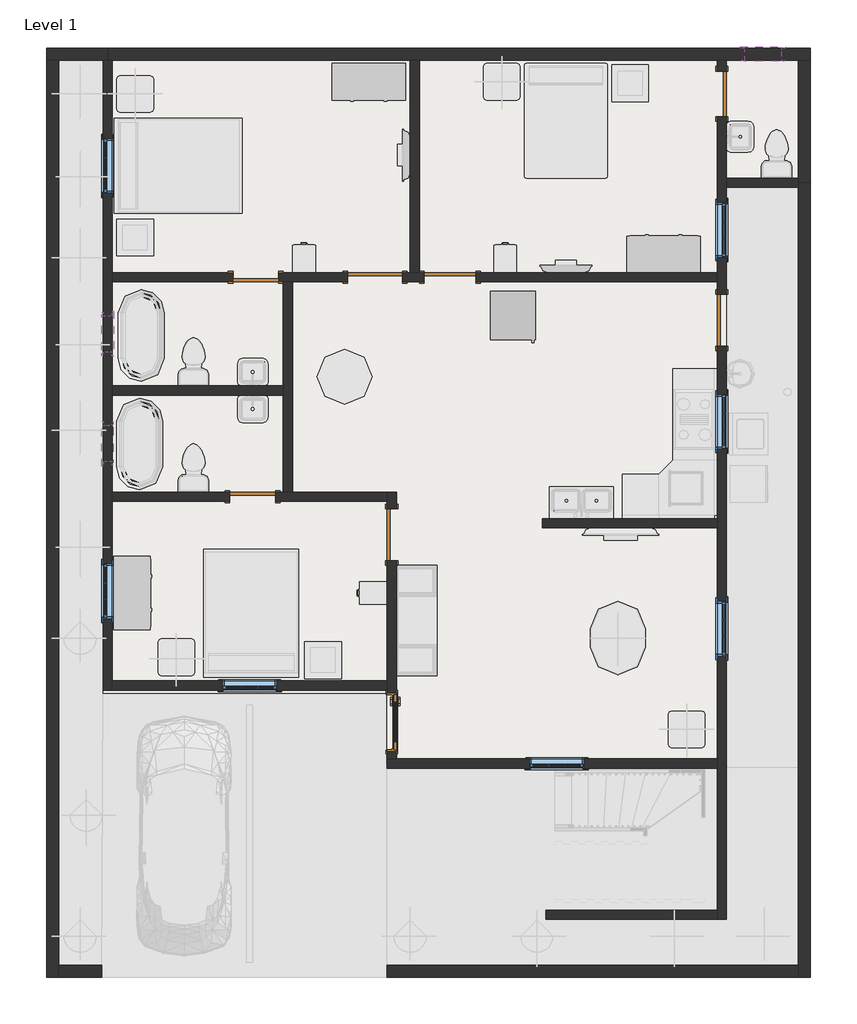
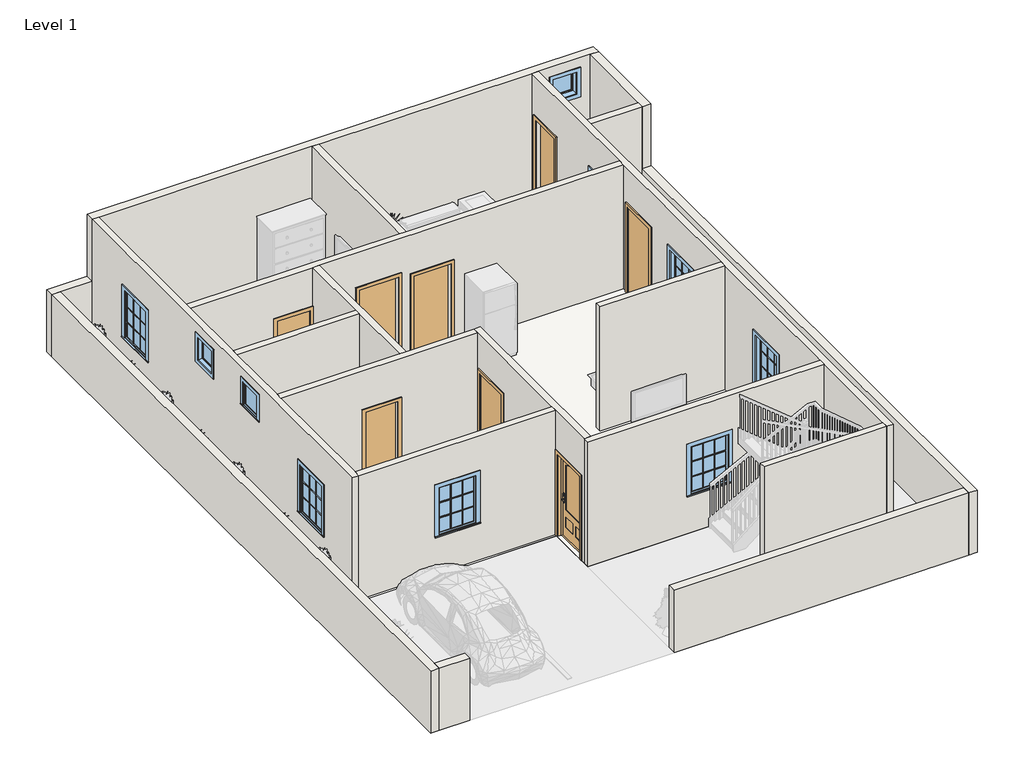
# One storey, part 1 of 3: 20 walls, 10 windows, 8 doors, 1 slab.
"""IFC4 building model written with IfcOpenShell, lengths in millimetres."""

from ifc_helpers import new_model, si_unit, frame, origin, origin_with_axes, place, context, project, spatial, polyline, outline, extrude, faceted_brep, transform, mapped, element, save
from components import door_5d363d20, door_255cab33, door_059fdd7e, door_706f0888, door_b6e9fca3, door_16372e1c, window_5c190c7e, window_e41d21a6, window_3d781103

model = new_model("IFC4")

# Units and contexts
model_context = context("Model", 3, world=origin())
ifc_project = project(units=[si_unit("LENGTHUNIT", "METRE", prefix="MILLI")], contexts=[model_context])

# Site, building, storey
site = spatial("IfcSite", under=ifc_project)
building = spatial("IfcBuilding", under=site)
storey = spatial("IfcBuildingStorey", under=building, Name="Level 1", Elevation=0.0)

# Doors
placement = place(None, origin())
door_shape = door_5d363d20(model_context)
element("IfcDoor", 1, ObjectType="36\" x 80\"", at=placement, inside=storey, context=model_context, shape_type="MappedRepresentation", body=[
    mapped(door_shape, transform((-6677.6504019, 2135.1007235, 0.0), x_axis=(0.0, 1.0, 0.0), y_axis=(-1.0, 0.0, 0.0), z_axis=(0.0, 0.0, 1.0))),
])
door_2_shape = door_255cab33(model_context)
element("IfcDoor", 2, ObjectType="Single-Flush : 30\" x 80\"", at=placement, inside=storey, context=model_context, shape_type="MappedRepresentation", body=[
    mapped(door_2_shape, transform((-8941.4254019, 9526.5007235, 0.0), x_axis=(1.0, 0.0, 0.0), y_axis=(0.0, 1.0, 0.0), z_axis=(0.0, 0.0, 1.0))),
])
element("IfcDoor", 3, ObjectType="Single-Flush : 30\" x 80\"", at=placement, inside=storey, context=model_context, shape_type="MappedRepresentation", body=[
    mapped(door_2_shape, transform((-1194.4254019, 12574.5007235, 0.0), x_axis=(0.0, 1.0, 0.0), y_axis=(-1.0, 0.0, 0.0), z_axis=(0.0, 0.0, 1.0))),
])
door_3_shape = door_059fdd7e(model_context)
element("IfcDoor", 4, ObjectType="Single-Flush : 30\" x 80\"", at=placement, inside=storey, context=model_context, shape_type="MappedRepresentation", body=[
    mapped(door_3_shape, transform((-8992.2254019, 5882.5032847, 0.0), x_axis=(1.0, 0.0, 0.0), y_axis=(0.0, 1.0, 0.0), z_axis=(0.0, 0.0, 1.0))),
])
door_4_shape = door_706f0888(model_context)
element("IfcDoor", 5, ObjectType="Single-Flush : 34\" x 80\"", at=placement, inside=storey, context=model_context, shape_type="MappedRepresentation", body=[
    mapped(door_4_shape, transform((-5715.6254019, 9526.5007235, 0.0), x_axis=(-1.0, 0.0, 0.0), y_axis=(0.0, -1.0, 0.0), z_axis=(0.0, 0.0, 1.0))),
])
door_5_shape = door_b6e9fca3(model_context)
element("IfcDoor", 6, ObjectType="Single-Flush : 34\" x 84\"", at=placement, inside=storey, context=model_context, shape_type="MappedRepresentation", body=[
    mapped(door_5_shape, transform((-6680.8254019, 5247.5032847, 0.0), x_axis=(0.0, 1.0, 0.0), y_axis=(-1.0, 0.0, 0.0), z_axis=(0.0, 0.0, 1.0))),
])
element("IfcDoor", 7, ObjectType="Single-Flush : 34\" x 84\"", at=placement, inside=storey, context=model_context, shape_type="MappedRepresentation", body=[
    mapped(door_5_shape, transform((-1194.4254019, 8815.3007235, 0.0), x_axis=(0.0, 1.0, 0.0), y_axis=(-1.0, 0.0, 0.0), z_axis=(0.0, 0.0, 1.0))),
])
door_6_shape = door_16372e1c(model_context)
element("IfcDoor", 8, ObjectType="Single-Flush : 36\" x 84\"", at=placement, inside=storey, context=model_context, shape_type="MappedRepresentation", body=[
    mapped(door_6_shape, transform((-6960.2254019, 9526.5007235, 0.0), x_axis=(1.0, 0.0, 0.0), y_axis=(0.0, 1.0, 0.0), z_axis=(0.0, 0.0, 1.0))),
])

# Slab
element("IfcSlab", 9, ObjectType="Generic - 12\"", at=placement, inside=storey, context=model_context, shape_type="SweptSolid", body=[
    extrude(outline(polyline([(278.7745981, 13336.5007235), (278.7745981, 11025.1007235), (-1118.2254019, 11025.1007235), (-1118.2254019, 1373.1007235), (-6757.0254019, 1373.1007235), (-6757.0254019, 2617.7007235), (-11481.4254019, 2617.7007235), (-11481.4254019, 13336.5007235), (278.7745981, 13336.5007235)])), frame((0.0, 0.0, -304.8), z_axis=(0.0, 0.0, 1.0), x_axis=(1.0, 0.0, 0.0)), (0.0, 0.0, 1.0), 304.8),
])

# Walls
element("IfcWall", 10, ObjectType="Generic - 8\"", at=placement, inside=storey, context=model_context, shape_type="Brep", body=[
    faceted_brep([(75.5745981, 13133.3007235, 0.0), (75.5745981, 11177.5007235, 0.0), (75.5745981, 11101.3007235, 0.0), (75.5745981, 11101.3007235, 1524.0), (75.5745981, 11025.1007235, 1524.0), (75.5745981, 11025.1007235, 3048.0), (75.5745981, 11177.5007235, 3048.0), (75.5745981, 13133.3007235, 3048.0), (278.7745981, 13133.3007235, 0.0), (278.7745981, 13133.3007235, 3048.0), (278.7745981, 11025.1007235, 3048.0), (278.7745981, 11025.1007235, 1524.0), (278.7745981, 11101.3007235, 1524.0), (278.7745981, 11101.3007235, 0.0)], [[[0, 1, 2, 3, 4, 5, 6, 7]], [[8, 9, 10, 11, 12, 13]], [[2, 1, 0, 8, 13]], [[0, 7, 9, 8]], [[3, 2, 13, 12]], [[11, 4, 3, 12]], [[5, 4, 11, 10]], [[7, 6, 5, 10, 9]]]),
])
element("IfcWall", 11, ObjectType="Generic - 8\"", at=placement, inside=storey, context=model_context, shape_type="Brep", body=[
    faceted_brep([(-11405.2254019, 13133.3007235, 0.0), (-11329.0254019, 13133.3007235, 0.0), (-6376.0254019, 13133.3007235, 0.0), (-6223.6254019, 13133.3007235, 0.0), (-1270.6254019, 13133.3007235, 0.0), (-1118.2254019, 13133.3007235, 0.0), (75.5745981, 13133.3007235, 0.0), (278.7745981, 13133.3007235, 0.0), (278.7745981, 13133.3007235, 3048.0), (75.5745981, 13133.3007235, 3048.0), (-1118.2254019, 13133.3007235, 3048.0), (-1270.6254019, 13133.3007235, 3048.0), (-6223.6254019, 13133.3007235, 3048.0), (-6376.0254019, 13133.3007235, 3048.0), (-11329.0254019, 13133.3007235, 3048.0), (-11481.4254019, 13133.3007235, 3048.0), (-11481.4254019, 13133.3007235, 1524.0), (-11405.2254019, 13133.3007235, 1524.0), (-203.8254019, 13133.3007235, 2768.6), (-203.8254019, 13133.3007235, 2159.0), (-813.4254019, 13133.3007235, 2159.0), (-813.4254019, 13133.3007235, 2768.6), (-11405.2254019, 13336.5007235, 0.0), (-11405.2254019, 13336.5007235, 1524.0), (-11481.4254019, 13336.5007235, 1524.0), (-11481.4254019, 13336.5007235, 3048.0), (278.7745981, 13336.5007235, 3048.0), (278.7745981, 13336.5007235, 0.0), (-203.8254019, 13336.5007235, 2768.6), (-813.4254019, 13336.5007235, 2768.6), (-813.4254019, 13336.5007235, 2159.0), (-203.8254019, 13336.5007235, 2159.0)], [[[0, 1, 2, 3, 4, 5, 6, 7, 8, 9, 10, 11, 12, 13, 14, 15, 16, 17], [18, 19, 20, 21]], [[22, 23, 24, 25, 26, 27], [28, 29, 30, 31]], [[7, 6, 5, 4, 3, 2, 1, 0, 22, 27]], [[8, 7, 27, 26]], [[19, 18, 28, 31]], [[20, 19, 31, 30]], [[21, 20, 30, 29]], [[18, 21, 29, 28]], [[0, 17, 23, 22]], [[16, 24, 23, 17]], [[16, 15, 25, 24]], [[15, 14, 13, 12, 11, 10, 9, 8, 26, 25]]]),
])
element("IfcWall", 12, ObjectType="INNER 6\"", at=placement, inside=storey, context=model_context, shape_type="Brep", body=[
    faceted_brep([(-6503.0254019, 9450.3007235, 0.0), (-6147.4254019, 9450.3007235, 0.0), (-6147.4254019, 9450.3007235, 2032.0), (-5283.8254019, 9450.3007235, 2032.0), (-5283.8254019, 9450.3007235, 0.0), (-1270.6254019, 9450.3007235, 0.0), (-1270.6254019, 9450.3007235, 3048.0), (-8331.8254019, 9450.3007235, 3048.0), (-8484.2254019, 9450.3007235, 3048.0), (-11329.0254019, 9450.3007235, 3048.0), (-11329.0254019, 9450.3007235, 0.0), (-9322.4254019, 9450.3007235, 0.0), (-9322.4254019, 9450.3007235, 2032.0), (-8560.4254019, 9450.3007235, 2032.0), (-8560.4254019, 9450.3007235, 0.0), (-8484.2254019, 9450.3007235, 0.0), (-8331.8254019, 9450.3007235, 0.0), (-7417.4254019, 9450.3007235, 0.0), (-7417.4254019, 9450.3007235, 2133.6), (-6503.0254019, 9450.3007235, 2133.6), (-6147.4254019, 9602.7007235, 2032.0), (-6147.4254019, 9602.7007235, 0.0), (-6223.6254019, 9602.7007235, 0.0), (-6376.0254019, 9602.7007235, 0.0), (-6503.0254019, 9602.7007235, 0.0), (-6503.0254019, 9602.7007235, 2133.6), (-7417.4254019, 9602.7007235, 2133.6), (-7417.4254019, 9602.7007235, 0.0), (-8560.4254019, 9602.7007235, 0.0), (-8560.4254019, 9602.7007235, 2032.0), (-9322.4254019, 9602.7007235, 2032.0), (-9322.4254019, 9602.7007235, 0.0), (-11329.0254019, 9602.7007235, 0.0), (-11329.0254019, 9602.7007235, 3048.0), (-6376.0254019, 9602.7007235, 3048.0), (-6223.6254019, 9602.7007235, 3048.0), (-1270.6254019, 9602.7007235, 3048.0), (-1270.6254019, 9602.7007235, 0.0), (-5283.8254019, 9602.7007235, 0.0), (-5283.8254019, 9602.7007235, 2032.0)], [[[0, 1, 2, 3, 4, 5, 6, 7, 8, 9, 10, 11, 12, 13, 14, 15, 16, 17, 18, 19]], [[20, 21, 22, 23, 24, 25, 26, 27, 28, 29, 30, 31, 32, 33, 34, 35, 36, 37, 38, 39]], [[11, 10, 32, 31]], [[17, 16, 15, 14, 28, 27]], [[38, 37, 5, 4]], [[24, 23, 22, 21, 1, 0]], [[10, 9, 33, 32]], [[6, 5, 37, 36]], [[25, 24, 0, 19]], [[26, 25, 19, 18]], [[27, 26, 18, 17]], [[29, 28, 14, 13]], [[30, 29, 13, 12]], [[31, 30, 12, 11]], [[2, 1, 21, 20]], [[3, 2, 20, 39]], [[4, 3, 39, 38]], [[9, 8, 7, 6, 36, 35, 34, 33]]]),
])
element("IfcWall", 13, ObjectType="INNER 6\"", at=placement, inside=storey, context=model_context, shape_type="SweptSolid", body=[
    extrude(outline(polyline([(-6223.6254019, 13133.3007235), (-6223.6254019, 9602.7007235), (-6376.0254019, 9602.7007235), (-6376.0254019, 13133.3007235), (-6223.6254019, 13133.3007235)])), origin_with_axes(), (0.0, 0.0, 1.0), 3048.0),
])
element("IfcWall", 14, ObjectType="INNER 6\"", at=placement, inside=storey, context=model_context, shape_type="Brep", body=[
    faceted_brep([(-1118.2254019, 12955.5007235, 2032.0), (-1118.2254019, 12955.5007235, 0.0), (-1118.2254019, 13133.3007235, 0.0), (-1118.2254019, 13133.3007235, 3048.0), (-1118.2254019, 11177.5007235, 3048.0), (-1118.2254019, 11025.1007235, 3048.0), (-1118.2254019, -1141.4992765, 3048.0), (-1118.2254019, -1141.4992765, 0.0), (-1118.2254019, 8383.5007235, 0.0), (-1118.2254019, 8383.5007235, 2133.6), (-1118.2254019, 9247.1007235, 2133.6), (-1118.2254019, 9247.1007235, 0.0), (-1118.2254019, 11025.1007235, 0.0), (-1118.2254019, 11177.5007235, 0.0), (-1118.2254019, 12193.5007235, 0.0), (-1118.2254019, 12193.5007235, 2032.0), (-1118.2254019, 3232.7671827, 2133.6), (-1118.2254019, 4147.1671827, 2133.6), (-1118.2254019, 4147.1671827, 914.4), (-1118.2254019, 3232.7671827, 914.4), (-1118.2254019, 6671.7339531, 2133.6), (-1118.2254019, 7586.1339531, 2133.6), (-1118.2254019, 7586.1339531, 914.4), (-1118.2254019, 6671.7339531, 914.4), (-1118.2254019, 9856.7007235, 2133.6), (-1118.2254019, 10771.1007235, 2133.6), (-1118.2254019, 10771.1007235, 914.4), (-1118.2254019, 9856.7007235, 914.4), (-1270.6254019, 13133.3007235, 0.0), (-1270.6254019, 12955.5007235, 0.0), (-1270.6254019, 12955.5007235, 2032.0), (-1270.6254019, 12193.5007235, 2032.0), (-1270.6254019, 12193.5007235, 0.0), (-1270.6254019, 9602.7007235, 0.0), (-1270.6254019, 9450.3007235, 0.0), (-1270.6254019, 9247.1007235, 0.0), (-1270.6254019, 9247.1007235, 2133.6), (-1270.6254019, 8383.5007235, 2133.6), (-1270.6254019, 8383.5007235, 0.0), (-1270.6254019, 5518.7671827, 0.0), (-1270.6254019, 5366.3671827, 0.0), (-1270.6254019, 1525.5007235, 0.0), (-1270.6254019, 1373.1007235, 0.0), (-1270.6254019, -989.0992765, 0.0), (-1270.6254019, -1141.4992765, 0.0), (-1270.6254019, -1141.4992765, 3048.0), (-1270.6254019, -989.0992765, 3048.0), (-1270.6254019, 1373.1007235, 3048.0), (-1270.6254019, 1525.5007235, 3048.0), (-1270.6254019, 5366.3671827, 3048.0), (-1270.6254019, 5518.7671827, 3048.0), (-1270.6254019, 9450.3007235, 3048.0), (-1270.6254019, 9602.7007235, 3048.0), (-1270.6254019, 13133.3007235, 3048.0), (-1270.6254019, 3232.7671827, 2133.6), (-1270.6254019, 3232.7671827, 914.4), (-1270.6254019, 4147.1671827, 914.4), (-1270.6254019, 4147.1671827, 2133.6), (-1270.6254019, 6671.7339531, 2133.6), (-1270.6254019, 6671.7339531, 914.4), (-1270.6254019, 7586.1339531, 914.4), (-1270.6254019, 7586.1339531, 2133.6), (-1270.6254019, 9856.7007235, 2133.6), (-1270.6254019, 9856.7007235, 914.4), (-1270.6254019, 10771.1007235, 914.4), (-1270.6254019, 10771.1007235, 2133.6)], [[[0, 1, 2, 3, 4, 5, 6, 7, 8, 9, 10, 11, 12, 13, 14, 15], [16, 17, 18, 19], [20, 21, 22, 23], [24, 25, 26, 27]], [[28, 29, 30, 31, 32, 33, 34, 35, 36, 37, 38, 39, 40, 41, 42, 43, 44, 45, 46, 47, 48, 49, 50, 51, 52, 53], [54, 55, 56, 57], [58, 59, 60, 61], [62, 63, 64, 65]], [[8, 7, 44, 43, 42, 41, 40, 39, 38]], [[2, 1, 29, 28]], [[14, 13, 12, 11, 35, 34, 33, 32]], [[3, 2, 28, 53]], [[7, 6, 45, 44]], [[36, 35, 11, 10]], [[37, 36, 10, 9]], [[38, 37, 9, 8]], [[30, 29, 1, 0]], [[31, 30, 0, 15]], [[32, 31, 15, 14]], [[55, 54, 16, 19]], [[56, 55, 19, 18]], [[57, 56, 18, 17]], [[54, 57, 17, 16]], [[59, 58, 20, 23]], [[60, 59, 23, 22]], [[61, 60, 22, 21]], [[58, 61, 21, 20]], [[63, 62, 24, 27]], [[64, 63, 27, 26]], [[65, 64, 26, 25]], [[62, 65, 25, 24]], [[6, 5, 4, 3, 53, 52, 51, 50, 49, 48, 47, 46, 45]]]),
])
element("IfcWall", 15, ObjectType="INNER 6\"", at=placement, inside=storey, context=model_context, shape_type="SweptSolid", body=[
    extrude(outline(polyline([(-4115.4254019, -989.0992765), (-1270.6254019, -989.0992765), (-1270.6254019, -1141.4992765), (-4115.4254019, -1141.4992765), (-4115.4254019, -989.0992765)])), origin_with_axes(), (0.0, 0.0, 1.0), 3048.0),
])
element("IfcWall", 16, ObjectType="INNER 6\"", at=placement, inside=storey, context=model_context, shape_type="Brep", body=[
    faceted_brep([(-1270.6254019, 1525.5007235, 0.0), (-6604.6254019, 1525.5007235, 0.0), (-6757.0254019, 1525.5007235, 0.0), (-6757.0254019, 1525.5007235, 3048.0), (-6604.6254019, 1525.5007235, 3048.0), (-1270.6254019, 1525.5007235, 3048.0), (-4394.8254019, 1525.5007235, 2133.6), (-4394.8254019, 1525.5007235, 914.4), (-3480.4254019, 1525.5007235, 914.4), (-3480.4254019, 1525.5007235, 2133.6), (-1270.6254019, 1373.1007235, 0.0), (-1270.6254019, 1373.1007235, 3048.0), (-6757.0254019, 1373.1007235, 3048.0), (-6757.0254019, 1373.1007235, 0.0), (-4394.8254019, 1373.1007235, 2133.6), (-3480.4254019, 1373.1007235, 2133.6), (-3480.4254019, 1373.1007235, 914.4), (-4394.8254019, 1373.1007235, 914.4)], [[[0, 1, 2, 3, 4, 5], [6, 7, 8, 9]], [[10, 11, 12, 13], [14, 15, 16, 17]], [[2, 1, 0, 10, 13]], [[0, 5, 11, 10]], [[3, 2, 13, 12]], [[7, 6, 14, 17]], [[8, 7, 17, 16]], [[9, 8, 16, 15]], [[6, 9, 15, 14]], [[5, 4, 3, 12, 11]]]),
])
element("IfcWall", 17, ObjectType="INNER 6\"", at=placement, inside=storey, context=model_context, shape_type="Brep", body=[
    faceted_brep([(-6604.6254019, 1525.5007235, 3048.0), (-6604.6254019, 1525.5007235, 0.0), (-6604.6254019, 1652.5007235, 0.0), (-6604.6254019, 1652.5007235, 2057.4), (-6604.6254019, 2617.7007235, 2057.4), (-6604.6254019, 2617.7007235, 0.0), (-6604.6254019, 4815.7032847, 0.0), (-6604.6254019, 4815.7032847, 2133.6), (-6604.6254019, 5679.3032847, 2133.6), (-6604.6254019, 5679.3032847, 0.0), (-6604.6254019, 5958.7032847, 0.0), (-6604.6254019, 5958.7032847, 3048.0), (-6757.0254019, 1525.5007235, 0.0), (-6757.0254019, 1525.5007235, 3048.0), (-6757.0254019, 2668.5007235, 3048.0), (-6757.0254019, 2820.9007235, 3048.0), (-6757.0254019, 5806.3032847, 3048.0), (-6757.0254019, 5958.7032847, 3048.0), (-6757.0254019, 5958.7032847, 0.0), (-6757.0254019, 5806.3032847, 0.0), (-6757.0254019, 5679.3032847, 0.0), (-6757.0254019, 5679.3032847, 2133.6), (-6757.0254019, 4815.7032847, 2133.6), (-6757.0254019, 4815.7032847, 0.0), (-6757.0254019, 2820.9007235, 0.0), (-6757.0254019, 2668.5007235, 0.0), (-6757.0254019, 2617.7007235, 0.0), (-6757.0254019, 2617.7007235, 2057.4), (-6757.0254019, 1652.5007235, 2057.4), (-6757.0254019, 1652.5007235, 0.0)], [[[0, 1, 2, 3, 4, 5, 6, 7, 8, 9, 10, 11]], [[12, 13, 14, 15, 16, 17, 18, 19, 20, 21, 22, 23, 24, 25, 26, 27, 28, 29]], [[1, 12, 29, 2]], [[18, 10, 9, 20, 19]], [[23, 6, 5, 26, 25, 24]], [[1, 0, 13, 12]], [[11, 10, 18, 17]], [[21, 20, 9, 8]], [[22, 21, 8, 7]], [[23, 22, 7, 6]], [[4, 27, 26, 5]], [[27, 4, 3, 28]], [[28, 3, 2, 29]], [[0, 11, 17, 16, 15, 14, 13]]]),
])
element("IfcWall", 18, ObjectType="INNER 6\"", at=placement, inside=storey, context=model_context, shape_type="Brep", body=[
    faceted_brep([(-8484.2254019, 9450.3007235, 0.0), (-8484.2254019, 7723.1007235, 0.0), (-8484.2254019, 7570.7007235, 0.0), (-8484.2254019, 5958.7032847, 0.0), (-8484.2254019, 5958.7032847, 3048.0), (-8484.2254019, 7570.7007235, 3048.0), (-8484.2254019, 7723.1007235, 3048.0), (-8484.2254019, 9450.3007235, 3048.0), (-8331.8254019, 9450.3007235, 0.0), (-8331.8254019, 9450.3007235, 3048.0), (-8331.8254019, 5958.7032847, 3048.0), (-8331.8254019, 5958.7032847, 0.0)], [[[0, 1, 2, 3, 4, 5, 6, 7]], [[8, 9, 10, 11]], [[3, 2, 1, 0, 8, 11]], [[0, 7, 9, 8]], [[4, 3, 11, 10]], [[7, 6, 5, 4, 10, 9]]]),
])
element("IfcWall", 19, ObjectType="INNER 6\"", at=placement, inside=storey, context=model_context, shape_type="Brep", body=[
    faceted_brep([(-6757.0254019, 5958.7032847, 0.0), (-8331.8254019, 5958.7032847, 0.0), (-8484.2254019, 5958.7032847, 0.0), (-8611.2254019, 5958.7032847, 0.0), (-8611.2254019, 5958.7032847, 2032.0), (-9373.2254019, 5958.7032847, 2032.0), (-9373.2254019, 5958.7032847, 0.0), (-11329.0254019, 5958.7032847, 0.0), (-11329.0254019, 5958.7032847, 3048.0), (-8484.2254019, 5958.7032847, 3048.0), (-8331.8254019, 5958.7032847, 3048.0), (-6757.0254019, 5958.7032847, 3048.0), (-8611.2254019, 5806.3032847, 2032.0), (-8611.2254019, 5806.3032847, 0.0), (-6757.0254019, 5806.3032847, 0.0), (-6757.0254019, 5806.3032847, 3048.0), (-11329.0254019, 5806.3032847, 3048.0), (-11329.0254019, 5806.3032847, 0.0), (-9373.2254019, 5806.3032847, 0.0), (-9373.2254019, 5806.3032847, 2032.0)], [[[0, 1, 2, 3, 4, 5, 6, 7, 8, 9, 10, 11]], [[12, 13, 14, 15, 16, 17, 18, 19]], [[18, 17, 7, 6]], [[14, 13, 3, 2, 1, 0]], [[8, 7, 17, 16]], [[0, 11, 15, 14]], [[4, 3, 13, 12]], [[5, 4, 12, 19]], [[6, 5, 19, 18]], [[11, 10, 9, 8, 16, 15]]]),
])
element("IfcWall", 20, ObjectType="INNER 6\"", at=placement, inside=storey, context=model_context, shape_type="SweptSolid", body=[
    extrude(outline(polyline([(-11329.0254019, 7723.1007235), (-8484.2254019, 7723.1007235), (-8484.2254019, 7570.7007235), (-11329.0254019, 7570.7007235), (-11329.0254019, 7723.1007235)])), origin_with_axes(), (0.0, 0.0, 1.0), 3048.0),
])
element("IfcWall", 21, ObjectType="INNER 6\"", at=placement, inside=storey, context=model_context, shape_type="SweptSolid", body=[
    extrude(outline(polyline([(0.0, -6757.0254019), (3048.0, -6757.0254019), (3048.0, -11329.0254019), (0.0, -11329.0254019), (0.0, -6757.0254019)]), holes=[polyline([(2133.6, -9500.2254019), (2133.6, -8585.8254019), (914.4, -8585.8254019), (914.4, -9500.2254019), (2133.6, -9500.2254019)])]), frame((0.0, 2668.5007235, 0.0), z_axis=(0.0, 1.0, 0.0), x_axis=(0.0, 0.0, 1.0)), (0.0, 0.0, 1.0), 152.4),
])
element("IfcWall", 22, ObjectType="INNER 6\"", at=placement, inside=storey, context=model_context, shape_type="Brep", body=[
    faceted_brep([(-11329.0254019, 2668.5007235, 0.0), (-11329.0254019, 2820.9007235, 0.0), (-11329.0254019, 5806.3032847, 0.0), (-11329.0254019, 5958.7032847, 0.0), (-11329.0254019, 7570.7007235, 0.0), (-11329.0254019, 7723.1007235, 0.0), (-11329.0254019, 9450.3007235, 0.0), (-11329.0254019, 9602.7007235, 0.0), (-11329.0254019, 13133.3007235, 0.0), (-11329.0254019, 13133.3007235, 3048.0), (-11329.0254019, 9602.7007235, 3048.0), (-11329.0254019, 9450.3007235, 3048.0), (-11329.0254019, 7723.1007235, 3048.0), (-11329.0254019, 7570.7007235, 3048.0), (-11329.0254019, 5958.7032847, 3048.0), (-11329.0254019, 5806.3032847, 3048.0), (-11329.0254019, 2820.9007235, 3048.0), (-11329.0254019, 2668.5007235, 3048.0), (-11329.0254019, 11837.9007235, 2133.6), (-11329.0254019, 11837.9007235, 914.4), (-11329.0254019, 10923.5007235, 914.4), (-11329.0254019, 10923.5007235, 2133.6), (-11329.0254019, 4770.8020041, 2133.6), (-11329.0254019, 4770.8020041, 914.4), (-11329.0254019, 3856.4020041, 914.4), (-11329.0254019, 3856.4020041, 2133.6), (-11329.0254019, 8281.9007235, 2768.6), (-11329.0254019, 8891.5007235, 2768.6), (-11329.0254019, 8891.5007235, 2159.0), (-11329.0254019, 8281.9007235, 2159.0), (-11329.0254019, 7069.5020041, 2768.6), (-11329.0254019, 7069.5020041, 2159.0), (-11329.0254019, 6459.9020041, 2159.0), (-11329.0254019, 6459.9020041, 2768.6), (-11481.4254019, 2668.5007235, 0.0), (-11481.4254019, 2668.5007235, 3048.0), (-11481.4254019, 13133.3007235, 3048.0), (-11481.4254019, 13133.3007235, 1524.0), (-11481.4254019, 13133.3007235, 0.0), (-11481.4254019, 11837.9007235, 2133.6), (-11481.4254019, 10923.5007235, 2133.6), (-11481.4254019, 10923.5007235, 914.4), (-11481.4254019, 11837.9007235, 914.4), (-11481.4254019, 4770.8020041, 2133.6), (-11481.4254019, 3856.4020041, 2133.6), (-11481.4254019, 3856.4020041, 914.4), (-11481.4254019, 4770.8020041, 914.4), (-11481.4254019, 8281.9007235, 2768.6), (-11481.4254019, 8281.9007235, 2159.0), (-11481.4254019, 8891.5007235, 2159.0), (-11481.4254019, 8891.5007235, 2768.6), (-11481.4254019, 7069.5020041, 2768.6), (-11481.4254019, 6459.9020041, 2768.6), (-11481.4254019, 6459.9020041, 2159.0), (-11481.4254019, 7069.5020041, 2159.0), (-11405.2254019, 13133.3007235, 0.0)], [[[0, 1, 2, 3, 4, 5, 6, 7, 8, 9, 10, 11, 12, 13, 14, 15, 16, 17], [18, 19, 20, 21], [22, 23, 24, 25], [26, 27, 28, 29], [30, 31, 32, 33]], [[34, 35, 36, 37, 38], [39, 40, 41, 42], [43, 44, 45, 46], [47, 48, 49, 50], [51, 52, 53, 54]], [[8, 7, 6, 5, 4, 3, 2, 1, 0, 34, 38, 55]], [[0, 17, 35, 34]], [[19, 18, 39, 42]], [[20, 19, 42, 41]], [[21, 20, 41, 40]], [[18, 21, 40, 39]], [[23, 22, 43, 46]], [[24, 23, 46, 45]], [[25, 24, 45, 44]], [[22, 25, 44, 43]], [[48, 47, 26, 29]], [[49, 48, 29, 28]], [[50, 49, 28, 27]], [[47, 50, 27, 26]], [[31, 30, 51, 54]], [[32, 31, 54, 53]], [[33, 32, 53, 52]], [[30, 33, 52, 51]], [[8, 55, 38, 37, 36, 9]], [[17, 16, 15, 14, 13, 12, 11, 10, 9, 36, 35]]]),
])
element("IfcWall", 23, ObjectType="INNER 6\"", at=placement, inside=storey, context=model_context, shape_type="SweptSolid", body=[
    extrude(outline(polyline([(-1270.6254019, 5366.3671827), (-4175.3206124, 5366.3671827), (-4175.3206124, 5518.7671827), (-1270.6254019, 5518.7671827), (-1270.6254019, 5366.3671827)])), origin_with_axes(), (0.0, 0.0, 1.0), 3048.0),
])
element("IfcWall", 24, ObjectType="INNER 6\"", at=placement, inside=storey, context=model_context, shape_type="Brep", body=[
    faceted_brep([(75.5745981, 11177.5007235, 3048.0), (75.5745981, 11177.5007235, 0.0), (-1118.2254019, 11177.5007235, 0.0), (-1118.2254019, 11177.5007235, 3048.0), (75.5745981, 11025.1007235, 0.0), (75.5745981, 11025.1007235, 1524.0), (75.5745981, 11025.1007235, 3048.0), (-1118.2254019, 11025.1007235, 3048.0), (-1118.2254019, 11025.1007235, 0.0), (75.5745981, 11101.3007235, 0.0)], [[[0, 1, 2, 3]], [[4, 5, 6, 7, 8]], [[2, 1, 9, 4, 8]], [[3, 2, 8, 7]], [[0, 6, 5, 4, 9, 1]], [[0, 3, 7, 6]]]),
])
element("IfcWall", 25, ObjectType="OUTER 5'", at=placement, inside=storey, context=model_context, shape_type="Brep", body=[
    faceted_brep([(-12421.2254019, 13133.3007235, 0.0), (-12218.0254019, 13133.3007235, 0.0), (-11481.4254019, 13133.3007235, 0.0), (-11405.2254019, 13133.3007235, 0.0), (-11405.2254019, 13133.3007235, 1524.0), (-12218.0254019, 13133.3007235, 1524.0), (-12421.2254019, 13133.3007235, 1524.0), (-12421.2254019, 13336.5007235, 0.0), (-12421.2254019, 13336.5007235, 1524.0), (-11405.2254019, 13336.5007235, 1524.0), (-11405.2254019, 13336.5007235, 0.0)], [[[0, 1, 2, 3, 4, 5, 6]], [[7, 8, 9, 10]], [[3, 2, 1, 0, 7, 10]], [[4, 3, 10, 9]], [[6, 5, 4, 9, 8]], [[0, 6, 8, 7]]]),
])
element("IfcWall", 26, ObjectType="OUTER 5'", at=placement, inside=storey, context=model_context, shape_type="SweptSolid", body=[
    extrude(outline(polyline([(-6757.0254019, -1903.4992765), (75.5745981, -1903.4992765), (75.5745981, -2106.6992765), (-6757.0254019, -2106.6992765), (-6757.0254019, -1903.4992765)])), origin_with_axes(), (0.0, 0.0, 1.0), 1524.0),
])
element("IfcWall", 27, ObjectType="OUTER 5'", at=placement, inside=storey, context=model_context, shape_type="Brep", body=[
    faceted_brep([(-12421.2254019, 13133.3007235, 0.0), (-12421.2254019, -2106.6992765, 0.0), (-12421.2254019, -2106.6992765, 1524.0), (-12421.2254019, 13133.3007235, 1524.0), (-12218.0254019, 13133.3007235, 0.0), (-12218.0254019, 13133.3007235, 1524.0), (-12218.0254019, -1903.4992765, 1524.0), (-12218.0254019, -2106.6992765, 1524.0), (-12218.0254019, -2106.6992765, 0.0), (-12218.0254019, -1903.4992765, 0.0)], [[[0, 1, 2, 3]], [[4, 5, 6, 7, 8, 9]], [[1, 0, 4, 9, 8]], [[3, 2, 7, 6, 5]], [[0, 3, 5, 4]], [[2, 1, 8, 7]]]),
])
element("IfcWall", 28, ObjectType="OUTER 5'", at=placement, inside=storey, context=model_context, shape_type="SweptSolid", body=[
    extrude(outline(polyline([(-12218.0254019, -1903.4992765), (-11506.8254019, -1903.4992765), (-11506.8254019, -2106.6992765), (-12218.0254019, -2106.6992765), (-12218.0254019, -1903.4992765)])), origin_with_axes(), (0.0, 0.0, 1.0), 1524.0),
])
element("IfcWall", 29, ObjectType="OUTER 5'", at=placement, inside=storey, context=model_context, shape_type="Brep", body=[
    faceted_brep([(75.5745981, 11101.3007235, 0.0), (75.5745981, 11025.1007235, 0.0), (75.5745981, -1903.4992765, 0.0), (75.5745981, -2106.6992765, 0.0), (75.5745981, -2106.6992765, 1524.0), (75.5745981, -1903.4992765, 1524.0), (75.5745981, 11101.3007235, 1524.0), (278.7745981, 11101.3007235, 0.0), (278.7745981, 11101.3007235, 1524.0), (278.7745981, -2106.6992765, 1524.0), (278.7745981, -2106.6992765, 0.0)], [[[0, 1, 2, 3, 4, 5, 6]], [[7, 8, 9, 10]], [[3, 2, 1, 0, 7, 10]], [[6, 5, 4, 9, 8]], [[0, 6, 8, 7]], [[4, 3, 10, 9]]]),
])

# Windows
window_shape = window_5c190c7e(model_context)
element("IfcWindow", 30, ObjectType="Casement 3x3 with Trim : 36\" x 48\"", at=placement, inside=storey, context=model_context, shape_type="MappedRepresentation", body=[
    mapped(window_shape, transform((-11405.2254019, 11380.7007235, 0.0), x_axis=(0.0, 1.0, 0.0), y_axis=(-1.0, 0.0, 0.0), z_axis=(0.0, 0.0, 1.0))),
])
element("IfcWindow", 31, ObjectType="Casement 3x3 with Trim : 36\" x 48\"", at=placement, inside=storey, context=model_context, shape_type="MappedRepresentation", body=[
    mapped(window_shape, transform((-11405.2254019, 4313.6020041, 0.0), x_axis=(0.0, 1.0, 0.0), y_axis=(-1.0, 0.0, 0.0), z_axis=(0.0, 0.0, 1.0))),
])
element("IfcWindow", 32, ObjectType="Casement 3x3 with Trim : 36\" x 48\"", at=placement, inside=storey, context=model_context, shape_type="MappedRepresentation", body=[
    mapped(window_shape, transform((-9043.0254019, 2744.7007235, 0.0), x_axis=(-1.0, 0.0, 0.0), y_axis=(0.0, -1.0, 0.0), z_axis=(0.0, 0.0, 1.0))),
])
element("IfcWindow", 33, ObjectType="Casement 3x3 with Trim : 36\" x 48\"", at=placement, inside=storey, context=model_context, shape_type="MappedRepresentation", body=[
    mapped(window_shape, transform((-3937.6254019, 1449.3007235, 0.0), x_axis=(-1.0, 0.0, 0.0), y_axis=(0.0, -1.0, 0.0), z_axis=(0.0, 0.0, 1.0))),
])
element("IfcWindow", 34, ObjectType="Casement 3x3 with Trim : 36\" x 48\"", at=placement, inside=storey, context=model_context, shape_type="MappedRepresentation", body=[
    mapped(window_shape, transform((-1194.4254019, 3689.9671827, 0.0), x_axis=(0.0, -1.0, 0.0), y_axis=(1.0, 0.0, 0.0), z_axis=(0.0, 0.0, 1.0))),
])
element("IfcWindow", 35, ObjectType="Casement 3x3 with Trim : 36\" x 48\"", at=placement, inside=storey, context=model_context, shape_type="MappedRepresentation", body=[
    mapped(window_shape, transform((-1194.4254019, 7128.9339531, 0.0), x_axis=(0.0, -1.0, 0.0), y_axis=(1.0, 0.0, 0.0), z_axis=(0.0, 0.0, 1.0))),
])
element("IfcWindow", 36, ObjectType="Casement 3x3 with Trim : 36\" x 48\"", at=placement, inside=storey, context=model_context, shape_type="MappedRepresentation", body=[
    mapped(window_shape, transform((-1194.4254019, 10313.9007235, 0.0), x_axis=(0.0, -1.0, 0.0), y_axis=(1.0, 0.0, 0.0), z_axis=(0.0, 0.0, 1.0))),
])
window_2_shape = window_e41d21a6(model_context)
element("IfcWindow", 37, ObjectType="Transom with Trim : 24\" x 24\"", at=placement, inside=storey, context=model_context, shape_type="MappedRepresentation", body=[
    mapped(window_2_shape, transform((-470.5254019, 13234.9007235, 0.0), x_axis=(1.0, 0.0, 0.0), y_axis=(0.0, 1.0, 0.0), z_axis=(0.0, 0.0, 1.0))),
])
window_3_shape = window_3d781103(model_context)
element("IfcWindow", 38, ObjectType="Transom with Trim : 24\" x 24\"", at=placement, inside=storey, context=model_context, shape_type="MappedRepresentation", body=[
    mapped(window_3_shape, transform((-11405.2254019, 8548.6007235, 0.0), x_axis=(0.0, -1.0, 0.0), y_axis=(1.0, 0.0, 0.0), z_axis=(0.0, 0.0, 1.0))),
])
element("IfcWindow", 39, ObjectType="Transom with Trim : 24\" x 24\"", at=placement, inside=storey, context=model_context, shape_type="MappedRepresentation", body=[
    mapped(window_3_shape, transform((-11405.2254019, 6802.8020041, 0.0), x_axis=(0.0, 1.0, 0.0), y_axis=(-1.0, 0.0, 0.0), z_axis=(0.0, 0.0, 1.0))),
])

save(model, "model.ifc")

# Revit data of these elements
# Type "36\" x 80\""
#   Type Mark = "8"
#   Assembly Code = "B2030100"
#   Analytic Construction = "French door, wood frame with single glass"
#   Threshold Offset [instance default] = 0' - 0 1/2"
#   Thickness = 0' - 1 3/8"
#   Thermal Resistance (R) = 1.0696 (h·ft²·°F)/BTU
#   Swing Angle [instance default] = 90.00°
#   Stiles = 0' - 4 3/4"
#   Rough Width = 3' - 2"
#   Rough Height = 6' - 9"
#   Radius = 1' - 8.05625"
#   Lock Rail = 0' - 7 1/8"
#   Height = 6' - 8"
#   Width = 3' - 0"
#   Heat Transfer Coefficient (U) = 0.9350 BTU/(h·ft²·°F)
#   Door Offset [instance default] = 0' - 0"
#   Bottom Rail = 0' - 9 1/2"
#   Threshold [instance default] = yes
#   Function = 1
#   Exterior Trim [instance default] = yes
#   Trim Material = Cherry
#   Threshold Material = Cherry
#   Panel Material = Cherry
#   Glazing = Glass
#   Frame Material = Cherry
#   Door Handle Material = Aluminum
#   Visual Light Transmittance = 0
#   Solar Heat Gain Coefficient = 0
#   Wall Closure = (empty or 0)
#   Construction Type = (empty or 0)
# Type "Single-Flush : 30\" x 80\""
#   Type Mark = "5"
#   Construction Type Id = "MDOOR"
#   Assembly Code = "C1020"
#   Analytic Construction = "Metal"
#   Thickness = 0' - 2"
#   Heat Transfer Coefficient (U) = 0.651978 BTU/(h·ft²·°F)
#   Height = 6' - 8"
#   Trim Projection Ext = 0' - 1"
#   Trim Projection Int = 0' - 1"
#   Trim Width = 0' - 3"
#   Width = 2' - 6"
#   Define Thermal Properties by = 1
#   Door Material = Door - Panel
#   Frame Material = Door - Frame
#   Visual Light Transmittance = 0
#   Solar Heat Gain Coefficient = 0
#   Function = (empty or 0)
#   Wall Closure = (empty or 0)
# Type "Single-Flush : 34\" x 80\""
#   Type Mark = "7"
#   Construction Type Id = "MDOOR"
#   Assembly Code = "C1020"
#   Analytic Construction = "Metal"
#   Thickness = 0' - 2"
#   Heat Transfer Coefficient (U) = 0.651978 BTU/(h·ft²·°F)
#   Height = 6' - 8"
#   Trim Projection Ext = 0' - 1"
#   Trim Projection Int = 0' - 1"
#   Trim Width = 0' - 3"
#   Width = 2' - 10"
#   Define Thermal Properties by = 1
#   Door Material = Door - Panel
#   Frame Material = Door - Frame
#   Visual Light Transmittance = 0
#   Solar Heat Gain Coefficient = 0
#   Function = (empty or 0)
#   Wall Closure = (empty or 0)
# Type "Single-Flush : 34\" x 84\""
#   Type Mark = "2"
#   Construction Type Id = "MDOOR"
#   Assembly Code = "C1020"
#   Analytic Construction = "Metal"
#   Thickness = 0' - 2"
#   Heat Transfer Coefficient (U) = 0.651978 BTU/(h·ft²·°F)
#   Height = 7' - 0"
#   Trim Projection Ext = 0' - 1"
#   Trim Projection Int = 0' - 1"
#   Trim Width = 0' - 3"
#   Width = 2' - 10"
#   Define Thermal Properties by = 1
#   Door Material = Door - Panel
#   Frame Material = Door - Frame
#   Visual Light Transmittance = 0
#   Solar Heat Gain Coefficient = 0
#   Function = (empty or 0)
#   Wall Closure = (empty or 0)
# Type "Single-Flush : 36\" x 84\""
#   Type Mark = "1"
#   Construction Type Id = "MDOOR"
#   Assembly Code = "C1020"
#   Analytic Construction = "Metal"
#   Thickness = 0' - 2"
#   Heat Transfer Coefficient (U) = 0.651978 BTU/(h·ft²·°F)
#   Height = 7' - 0"
#   Trim Projection Ext = 0' - 1"
#   Trim Projection Int = 0' - 1"
#   Trim Width = 0' - 3"
#   Width = 3' - 0"
#   Define Thermal Properties by = 1
#   Door Material = Door - Panel
#   Frame Material = Door - Frame
#   Visual Light Transmittance = 0
#   Solar Heat Gain Coefficient = 0
#   Function = (empty or 0)
#   Wall Closure = (empty or 0)
# Type "Generic - 12\""
#   Assembly Code = "B1010"
#   Function = 0
#   Layers, outside or top first: 1' - 0" no material (function 1)
# Type "Generic - 8\""
#   Assembly Code = "B2010"
#   Layers, outside or top first: 0' - 8" "Brick, Common" (function 1)
# Type "INNER 6\""
#   Assembly Code = "B2010"
#   Layers, outside or top first: 0' - 6" "Brick, Common" (function 1)
# Type "OUTER 5'"
#   Assembly Code = "B2010"
#   Layers, outside or top first: 0' - 8" "Birch" (function 1)
# Type "Casement 3x3 with Trim : 36\" x 48\""
#   Type Mark = "10"
#   Construction Type Id = "GSP4R"
#   Assembly Code = "B2020100"
#   Analytic Construction = "1/8 in Pilkington single glazing"
#   Visual Light Transmittance = 0.9
#   Solar Heat Gain Coefficient = 0.78
#   Heat Transfer Coefficient (U) = 0.6496 BTU/(h·ft²·°F)
#   Height = 4' - 0"
#   Default Sill Height = 3' - 0"
#   Trim Projection - Ext. = 0' - 0 1/2"
#   Trim Projection - Int. = 0' - 0 3/4"
#   Trim Width - Exterior = 0' - 3 1/2"
#   Trim Width - Interior = 0' - 3 1/2"
#   Width = 3' - 0"
#   Window Inset = 0' - 0 3/4"
#   Define Thermal Properties by = 1
#   Glass Pane Material = Glass
#   Sash Material = Sash
#   Trim Exterior Material = Trim
#   Trim Interior Material = Trim
#   Wall Closure = (empty or 0)
# Type "Transom with Trim : 24\" x 24\""
#   Type Mark = "13"
#   Construction Type Id = "GSP4R"
#   Assembly Code = "B2020100"
#   Analytic Construction = "1/8 in Pilkington single glazing"
#   Visual Light Transmittance = 0.9
#   Solar Heat Gain Coefficient = 0.78
#   Heat Transfer Coefficient (U) = 0.6496 BTU/(h·ft²·°F)
#   Height = 2' - 0"
#   Default Sill Height = 7' - 1"
#   Trim Projection - Ext. = 0' - 0 1/2"
#   Trim Projection - Int. = 0' - 0 3/4"
#   Trim Width - Exterior = 0' - 3 1/2"
#   Trim Width - Interior = 0' - 3 1/2"
#   Width = 2' - 0"
#   Window Inset = 0' - 0 3/4"
#   Define Thermal Properties by = 1
#   Glass Pane Material = Glass
#   Sash Material = Sash
#   Trim Exterior Material = Trim
#   Trim Interior Material = Trim
#   Wall Closure = (empty or 0)
# Element 1 (IfcDoor, "36\" x 80\"")
#   Threshold Offset = 0' - 0 1/2"
#   Swing Angle = 90.00°
#   Door Offset = 0' - 0"
#   Threshold = yes
#   Exterior Trim = yes
#   Phase Created = New Construction
#   Materials on its faces: "Cherry", "Aluminum", "Glass"
# Elements 2, 3, 4 (IfcDoor, "Single-Flush : 30\" x 80\"")
#   Phase Created = New Construction
#   Materials on its faces: "Door - Frame", "Door - Panel"
# Element 5 (IfcDoor, "Single-Flush : 34\" x 80\"")
#   Phase Created = New Construction
#   Materials on its faces: "Door - Frame", "Door - Panel"
# Elements 6, 7 (IfcDoor, "Single-Flush : 34\" x 84\"")
#   Phase Created = New Construction
#   Materials on its faces: "Door - Frame", "Door - Panel"
# Element 8 (IfcDoor, "Single-Flush : 36\" x 84\"")
#   Phase Created = New Construction
#   Materials on its faces: "Door - Frame", "Door - Panel"
# Element 9 (IfcSlab, "Generic - 12\"")
#   Height Offset From Level = 0' - 0"
#   Phase Created = New Construction
#   Materials on its faces: "Default Floor"
# Elements 10, 11 (IfcWall, "Generic - 8\"")
#   Top Offset = 0' - 0"
#   Base Offset = 0' - 0"
#   Unconnected Height = 10' - 0"
#   wall height = 10' - 0"
#   Phase Created = New Construction
#   Base Constraint = Level 1
#   Materials on its faces: "Brick, Common"
# Elements 12, 13, 14, 15, 16, 17, 18, 19, 20, 21, 22, 23, 24 (IfcWall, "INNER 6\"")
#   Top Offset = 0' - 0"
#   Base Offset = 0' - 0"
#   Unconnected Height = 10' - 0"
#   wall height = 10' - 0"
#   Phase Created = New Construction
#   Base Constraint = Level 1
#   Materials on its faces: "Brick, Common"
# Elements 25, 26, 27, 28, 29 (IfcWall, "OUTER 5'")
#   Top Offset = 0' - 0"
#   Base Offset = 0' - 0"
#   Unconnected Height = 5' - 0"
#   wall height = 5' - 0"
#   Phase Created = New Construction
#   Base Constraint = Level 1
#   Materials on its faces: "Birch"
# Element 30 (IfcWindow, "Casement 3x3 with Trim : 36\" x 48\"")
#   Mark = "1"
#   Phase Created = New Construction
#   Materials on its faces: "Sash", "Glass", "Trim"
# Element 31 (IfcWindow, "Casement 3x3 with Trim : 36\" x 48\"")
#   Mark = "2"
#   Phase Created = New Construction
#   Materials on its faces: "Sash", "Glass", "Trim"
# Element 32 (IfcWindow, "Casement 3x3 with Trim : 36\" x 48\"")
#   Mark = "3"
#   Phase Created = New Construction
#   Materials on its faces: "Sash", "Glass", "Trim"
# Element 33 (IfcWindow, "Casement 3x3 with Trim : 36\" x 48\"")
#   Mark = "4"
#   Phase Created = New Construction
#   Materials on its faces: "Sash", "Glass", "Trim"
# Element 34 (IfcWindow, "Casement 3x3 with Trim : 36\" x 48\"")
#   Mark = "5"
#   Phase Created = New Construction
#   Materials on its faces: "Sash", "Glass", "Trim"
# Element 35 (IfcWindow, "Casement 3x3 with Trim : 36\" x 48\"")
#   Mark = "6"
#   Phase Created = New Construction
#   Materials on its faces: "Sash", "Glass", "Trim"
# Element 36 (IfcWindow, "Casement 3x3 with Trim : 36\" x 48\"")
#   Mark = "7"
#   Phase Created = New Construction
#   Materials on its faces: "Sash", "Glass", "Trim"
# Element 37 (IfcWindow, "Transom with Trim : 24\" x 24\"")
#   Mark = "8"
#   Phase Created = New Construction
#   Materials on its faces: "Sash", "Trim", "Glass"
# Element 38 (IfcWindow, "Transom with Trim : 24\" x 24\"")
#   Mark = "9"
#   Phase Created = New Construction
#   Materials on its faces: "Sash", "Trim", "Glass"
# Element 39 (IfcWindow, "Transom with Trim : 24\" x 24\"")
#   Mark = "10"
#   Phase Created = New Construction
#   Materials on its faces: "Sash", "Trim", "Glass"
# Materials
#   "Cherry": class "Wood", colour RGB 226 177 128, transparency 0, Description = "Prunus Serotina", Cost = 0
#   "Glass": class "Glass", colour RGB 0 128 192, transparency 0.75, Description = "Soda Lime Glass", Cost = 0
#   "Aluminum": class "Metal", colour RGB 247 247 247, transparency 0, Description = "Aluminum 6061", Cost = 0
#   "Door - Panel": class "Wood", colour RGB 210 159 95, transparency 0
#   "Door - Frame": colour RGB 118 70 51, transparency 0
#   "Brick, Common": class "Masonry", colour RGB 170 98 104, transparency 0, Description = "Common brick", Cost = 0
#   "Birch": class "Wood", colour RGB 224 178 126, transparency 0, Description = "Betula Alleghaniensis", Cost = 0
#   "Sash": class "Wood", colour RGB 224 178 126, transparency 0
#   "Trim": class "Wood", colour RGB 224 178 126, transparency 0
#   "Default Floor": colour RGB 128 128 128, transparency 0
# Room at (-8610.825, 11103.528) mm, phase "New Construction", upper level "Level 1", upper offset 10' - 0", lower offset 0' - 0"
#   Number = "1"
#   Name = "BEDROOM"
# Room at (-3618.875, 11255.928) mm, phase "New Construction", upper level "Level 1", upper offset 10' - 0", lower offset 0' - 0"
#   Number = "2"
#   Name = "BEDROOM"
# Room at (-8787.337, 4247.824) mm, phase "New Construction", upper level "Level 1", upper offset 10' - 0", lower offset 0' - 0"
#   Number = "3"
#   Name = "GUEST ROOM"
# Room at (-9974.133, 8422.531) mm, phase "New Construction", upper level "Level 1", upper offset 10' - 0", lower offset 0' - 0"
#   Number = "4"
#   Name = "BATHROOM"
# Room at (-9974.133, 6419.637) mm, phase "New Construction", upper level "Level 1", upper offset 10' - 0", lower offset 0' - 0"
#   Number = "5"
#   Name = "BATHROOM"
# Room at (-3795.387, 3469.303) mm, phase "New Construction", upper level "Level 1", upper offset 10' - 0", lower offset 0' - 0"
#   Number = "6"
#   Name = "LIVING HALL"
# Room at (-490.85, 11919.359) mm, phase "New Construction", upper level "Level 1", upper offset 10' - 0", lower offset 0' - 0"
#   Number = "7"
#   Name = "TOILET"
# Room at (-5051.767, 7681.792) mm, phase "New Construction", upper level "Level 1", upper offset 10' - 0", lower offset 0' - 0"
#   Number = "8"
